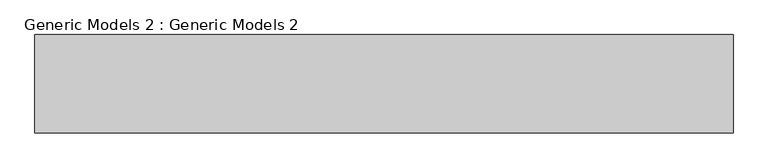
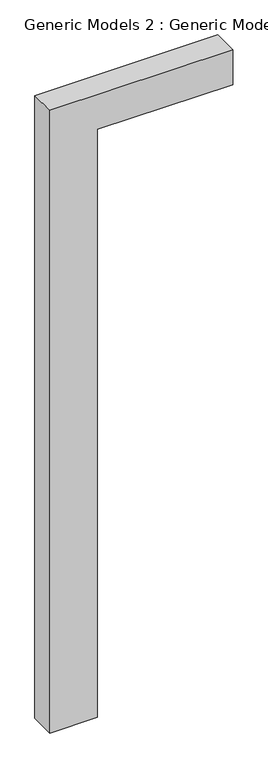
"""IFC4 building model written with IfcOpenShell, lengths in millimetres: proxy geometry, Generic Models 2 : Generic Models 2."""

from ifc_helpers import new_model, si_unit, frame, origin, place, context, project, spatial, polyline, outline, extrude, source, transform, mapped, element, save


def generic_models_2_generic_models_2_70f3bfce(model_context):
    return source(origin(), model_context, "Body", "SweptSolid", [
        extrude(outline(polyline([(7669.779075, 6619.47371), (7669.779075, 8222.8050525), (8107.2088974, 8222.8050525), (8107.2088974, 6054.6244585), (304.8, 6054.6244585), (304.8, 6619.47371), (7669.779075, 6619.47371)])), frame((0.0, -13806.7073314, 0.0), z_axis=(0.0, 1.0, 0.0), x_axis=(0.0, 0.0, 1.0)), (0.0, 0.0, 1.0), 304.8),
    ])


if __name__ == "__main__":
    model = new_model("IFC4")
    model_context = context("Model", 3, world=origin())
    ifc_project = project(units=[si_unit("LENGTHUNIT", "METRE", prefix="MILLI")], contexts=[model_context])
    site = spatial("IfcSite", under=ifc_project)
    building = spatial("IfcBuilding", under=site)
    placement = place(None, origin())
    generic_models_2_generic_models_2_shape = generic_models_2_generic_models_2_70f3bfce(model_context)
    element("IfcBuildingElementProxy", 1, Name="Generic Models 2 : Generic Models 2", ObjectType="Generic Models 2 : Generic Models 2", at=placement, inside=building, context=model_context, shape_type="MappedRepresentation", body=[
        mapped(generic_models_2_generic_models_2_shape, transform((0.0, 0.0, 0.0), x_axis=(1.0, 0.0, 0.0), y_axis=(0.0, 1.0, 0.0), z_axis=(0.0, 0.0, 1.0))),
    ])
    save(model, "model.ifc")

# Revit data of these elements
# Element 1 (IfcBuildingElementProxy, "Generic Models 2 : Generic Models 2")
#   Materials on its faces: "Clad - White"
# Materials
#   "Clad - White": class "Wood", colour RGB 242 242 238, transparency 0, Cost = 0
